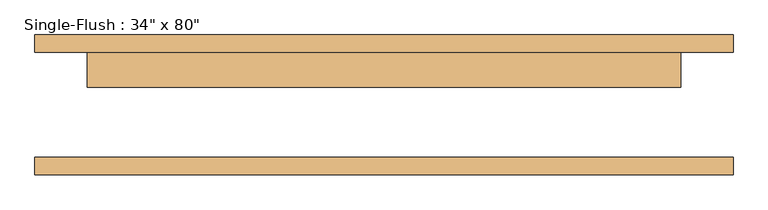
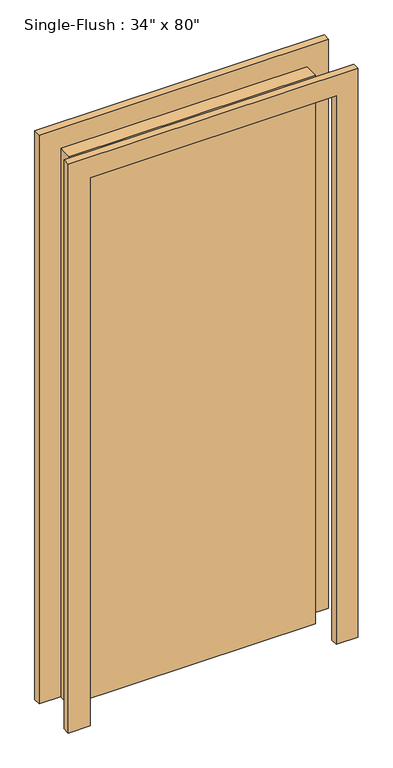
"""IFC4 building model written with IfcOpenShell, lengths in millimetres: door geometry."""

from ifc_helpers import new_model, si_unit, frame, origin, origin_with_axes, place, context, project, spatial, polyline, outline, extrude, source, transform, mapped, element, save


def door_56e8e0a9(model_context):
    return source(origin(), model_context, "Body", "SweptSolid", [
        extrude(outline(polyline([(2108.2, -508.0), (0.0, -508.0), (0.0, -431.8), (2032.0, -431.8), (2032.0, 431.8), (0.0, 431.8), (0.0, 508.0), (2108.2, 508.0), (2108.2, -508.0)])), frame((0.0, 76.2, 0.0), z_axis=(0.0, 1.0, 0.0), x_axis=(0.0, 0.0, 1.0)), (0.0, 0.0, 1.0), 25.4),
        extrude(outline(polyline([(2108.2, 508.0), (2108.2, -508.0), (0.0, -508.0), (0.0, -431.8), (2032.0, -431.8), (2032.0, 431.8), (0.0, 431.8), (0.0, 508.0), (2108.2, 508.0)])), frame((0.0, -101.6, 0.0), z_axis=(0.0, 1.0, 0.0), x_axis=(0.0, 0.0, 1.0)), (0.0, 0.0, 1.0), 25.4),
        extrude(outline(polyline([(431.8, 25.4), (-431.8, 25.4), (-431.8, 76.2), (431.8, 76.2), (431.8, 25.4)])), origin_with_axes(), (0.0, 0.0, 1.0), 2032.0),
    ])


if __name__ == "__main__":
    model = new_model("IFC4")
    model_context = context("Model", 3, world=origin())
    ifc_project = project(units=[si_unit("LENGTHUNIT", "METRE", prefix="MILLI")], contexts=[model_context])
    site = spatial("IfcSite", under=ifc_project)
    building = spatial("IfcBuilding", under=site)
    placement = place(None, origin())
    door_shape = door_56e8e0a9(model_context)
    element("IfcDoor", 1, ObjectType="Single-Flush : 34\" x 80\"", at=placement, inside=building, context=model_context, shape_type="MappedRepresentation", body=[
        mapped(door_shape, transform((0.0, 0.0, 0.0), x_axis=(1.0, 0.0, 0.0), y_axis=(0.0, 1.0, 0.0), z_axis=(0.0, 0.0, 1.0))),
    ])
    save(model, "model.ifc")

# Revit data of these elements
# Type "Single-Flush : 34\" x 80\""
#   Type Mark = "7"
#   Construction Type Id = "MDOOR"
#   Assembly Code = "C1020"
#   Analytic Construction = "Metal"
#   Thickness = 0' - 2"
#   Heat Transfer Coefficient (U) = 0.651978 BTU/(h·ft²·°F)
#   Height = 6' - 8"
#   Trim Projection Ext = 0' - 1"
#   Trim Projection Int = 0' - 1"
#   Trim Width = 0' - 3"
#   Width = 2' - 10"
#   Define Thermal Properties by = 1
#   Door Material = Door - Panel
#   Frame Material = Door - Frame
#   Visual Light Transmittance = 0
#   Solar Heat Gain Coefficient = 0
#   Function = (empty or 0)
#   Wall Closure = (empty or 0)
# Element 1 (IfcDoor, "Single-Flush : 34\" x 80\"")
#   Materials on its faces: "Door - Frame", "Door - Panel"
# Materials
#   "Door - Panel": class "Wood", colour RGB 210 159 95, transparency 0
#   "Door - Frame": colour RGB 118 70 51, transparency 0
